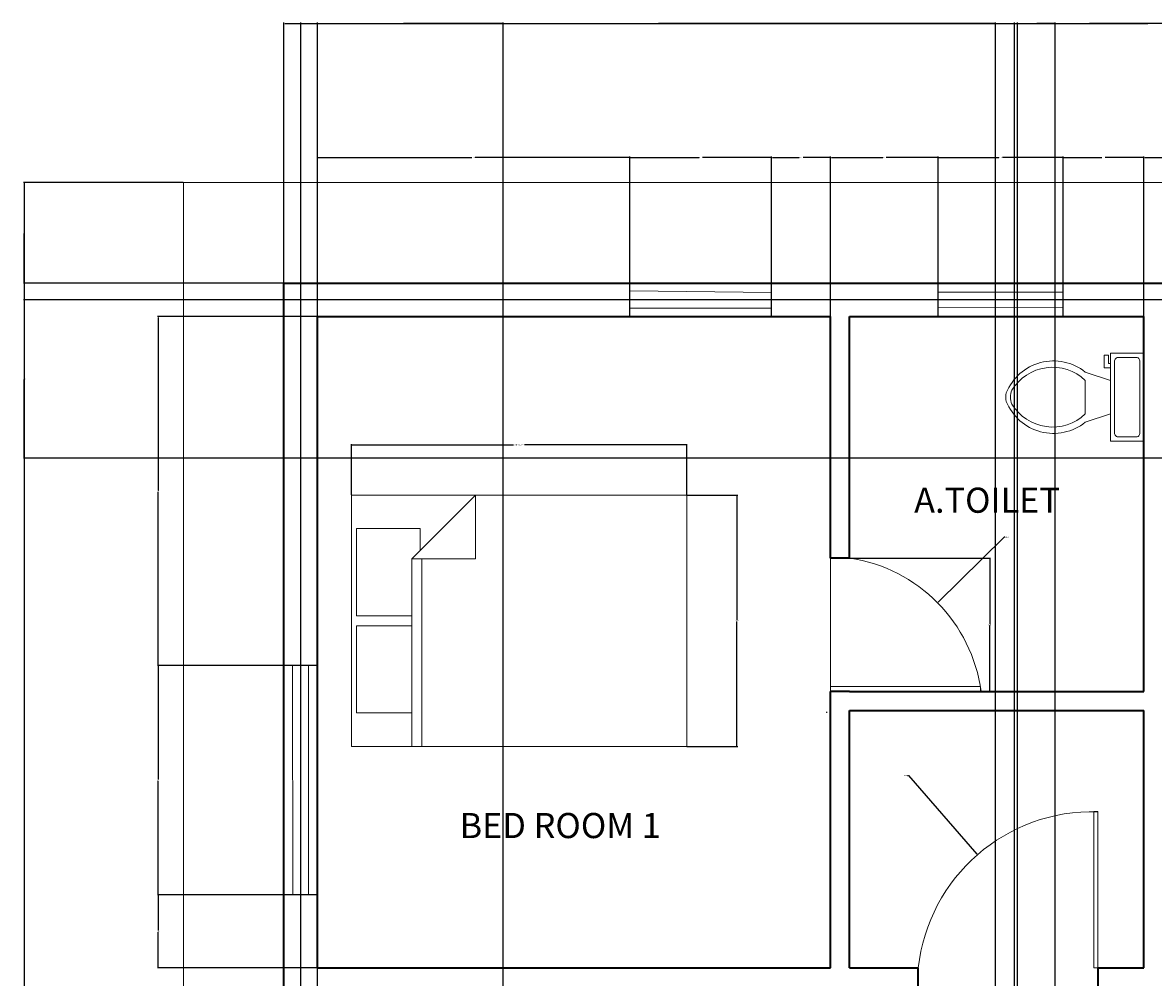
# Model space of a CAD drawing. Units: inches. Extents: x 4700 to 5209, y 8078 to 8754.
# Tile 4 of 5: x 4700 to 4970, y 8526 to 8754. Entities that reach past the tile are written whole.
import ezdxf

# ---------------------------------------------------------------- set-up
doc = ezdxf.new("R2010")
doc.units = ezdxf.units.IN
for name, color, linetype, lineweight in [('A-ANNO-DIMS', 2, 'Continuous', 18), ('A-AREA-IDEN', 7, 'Continuous', 18), ('A-DOOR', 3, 'Continuous', 18), ('A-FLOR-FIXT', 9, 'Continuous', 18), ('A-FURN', 8, 'Continuous', 18), ('A-GLAZ', 4, 'Continuous', 18), ('A-WALL', 7, 'Continuous', 35), ('C-PROP', 8, 'Continuous', 18)]:
    doc.layers.add(name, color=color, linetype=linetype, lineweight=lineweight)
doc.styles.get("Standard").update_dxf_attribs({"font": 'arial.ttf'})
doc.dimstyles.get("Standard").update_dxf_attribs({"dimtxt": 0.18, "dimasz": 0.18, "dimexe": 0.18, "dimexo": 0.0625, "dimgap": 0.09, "dimtad": 0, "dimtih": 1, "dimtoh": 1, "dimdec": 4, "dimzin": 0, "dimdsep": 46, "dimtxsty": 'Standard', "dimcen": 0.09, "dimadec": 0, "dimazin": 0, "dimtfac": 1, "dimtdec": 4, "dimtofl": 0, "dimtmove": 0, "dimatfit": 3, "dimfxl": 1, "dimtolj": 1, "dimtzin": 0, "dimarcsym": 0})

# ---------------------------------------------------------------- blocks, each defined once
blk = doc.blocks.new('Bed - Queen')
for p, q in [((0, -80.00003), (0, 0)), ((0, 0), (59.99999, 0)), ((59.99999, 0), (59.99999, -80.00003)), ((7.99999, -1.2), (28.79998, -1.2)), ((7.99999, -14.4), (7.99999, -1.2)), ((28.79998, -1.2), (28.79998, -14.4)), ((31.19999, -1.2), (51.99999, -1.2)), ((31.19999, -14.4), (31.19999, -1.2)), ((51.99999, -1.2), (51.99999, -16.4)), ((0, -14.4), (44.8, -14.4)), ((59.99999, -29.6), (44.8, -14.4)), ((44.8, -14.4), (44.8, -29.6)), ((44.8, -16.8), (0, -16.8)), ((51.99999, -16.4), (46.79936, -16.4)), ((44.8, -29.6), (59.99999, -29.6)), ((59.99999, -80.00003), (0, -80.00003))]:
    blk.add_line(p, q)
blk = doc.blocks.new('Toilet - top')
for p, q in [((9.5, -6), (9.5, -2)), ((-8, -8.5), (-8, -8)), ((-7, -8), (-7, -9.5)), ((-4, -8), (-6, -14)), ((4, -8), (6, -14)), ((-10, -8.5), (-8, -8.5)), ((-10, -9.5), (-10, -8.5)), ((-7, -9.5), (-10, -9.5)), ((4, -14), (-4, -14))]:
    blk.add_line(p, q)
blk.add_lwpolyline([(10.5, -8), (10.5, 0), (-10.5, 0), (-10.5, -8)], close=True)
for points in [[(-9.5, -2), (-9.5, -6)], [(8.5, -1), (-8.5, -1)], [(-8.5, -7), (8.5, -7)]]:
    blk.add_lwpolyline(points)
for centre, radius, start, end in [((-8.62, -1.88), 0.884, 81.8699, 188.1301), ((8.62, -1.88), 0.884, 351.8699, 98.1301), ((-8.62, -6.12), 0.884, 171.8699, 278.1301), ((8.62, -6.12), 0.884, 261.8699, 8.1301), ((3.52, -21.58), 12.17, 141.4691, 247.9714), ((4.2, -21.82), 11.33, 136.3677, 238.9468), ((-3.52, -21.58), 12.17, 292.0284, 38.5307), ((-4.2, -21.82), 11.33, 301.053, 43.6321), ((0, -27.88), 4, 245.7318, 294.2682), ((0, -29), 4, 254.8605, 285.1395)]:
    blk.add_arc(centre, radius, start, end)
blk = doc.blocks.new('*D6')
at = {"layer": 'A-ANNO-DIMS', "color": 0, "lineweight": -2, "transparency": 16777216}
for p, q in [((4778.93, 8641.19), (4778.93, 8653.31)), ((4779.11, 8653.13), (4817.62, 8653.13)), ((4858.75, 8653.13), (4820.23, 8653.13)), ((4858.93, 8641.19), (4858.93, 8653.31))]:
    blk.add_line(p, q, dxfattribs=at)
at = {"layer": 'A-ANNO-DIMS', "color": 0, "transparency": 16777216}
for points in [[(4779.11, 8653.16), (4779.11, 8653.1), (4778.93, 8653.13)], [(4858.75, 8653.16), (4858.75, 8653.1), (4858.93, 8653.13)]]:
    blk.add_solid(points, dxfattribs=at)
at = {"layer": 'Defpoints', "color": 0, "transparency": 16777216}
for p in [(4778.93, 8653.13), (4778.93, 8641.13), (4858.93, 8641.13)]:
    blk.add_point(p, dxfattribs=at)
at = {"layer": 'A-ANNO-DIMS', "color": 0, "transparency": 16777216, "insert": (4818.93, 8653.13), "char_height": 0.18, "attachment_point": 5}
blk.add_mtext('\\A1;QUEEN BED 80 TYP.', dxfattribs=at)
blk = doc.blocks.new('*D7')
at = {"layer": 'A-ANNO-DIMS', "color": 0, "lineweight": -2, "transparency": 16777216}
for p, q in [((4858.99, 8641.13), (4871.11, 8641.13)), ((4870.93, 8640.95), (4870.93, 8611.31)), ((4870.93, 8581.31), (4870.93, 8610.95)), ((4858.99, 8581.13), (4871.11, 8581.13))]:
    blk.add_line(p, q, dxfattribs=at)
at = {"layer": 'A-ANNO-DIMS', "color": 0, "transparency": 16777216}
for points in [[(4870.9, 8640.95), (4870.96, 8640.95), (4870.93, 8641.13)], [(4870.9, 8581.31), (4870.96, 8581.31), (4870.93, 8581.13)]]:
    blk.add_solid(points, dxfattribs=at)
at = {"layer": 'Defpoints', "color": 0, "transparency": 16777216}
for p in [(4858.93, 8641.13), (4870.93, 8641.13), (4858.93, 8581.13)]:
    blk.add_point(p, dxfattribs=at)
at = {"layer": 'A-ANNO-DIMS', "color": 0, "transparency": 16777216, "insert": (4870.93, 8611.13), "char_height": 0.18, "attachment_point": 5}
blk.add_mtext('\\A1;60 TYP.', dxfattribs=at)
blk = doc.blocks.new('*D15')
at = {"layer": 'A-ANNO-DIMS', "color": 0, "lineweight": -2, "transparency": 16777216}
for p, q in [((4738.72, 8715.75), (4700.6, 8715.75)), ((4700.78, 8715.57), (4700.78, 8415.93)), ((4700.78, 8115.93), (4700.78, 8415.57)), ((4738.72, 8115.75), (4700.6, 8115.75))]:
    blk.add_line(p, q, dxfattribs=at)
at = {"layer": 'A-ANNO-DIMS', "color": 0, "transparency": 16777216}
for points in [[(4700.75, 8715.57), (4700.81, 8715.57), (4700.78, 8715.75)], [(4700.75, 8115.93), (4700.81, 8115.93), (4700.78, 8115.75)]]:
    blk.add_solid(points, dxfattribs=at)
at = {"layer": 'Defpoints', "color": 0, "transparency": 16777216}
for p in [(4700.78, 8715.75), (4738.78, 8715.75), (4738.78, 8115.75)]:
    blk.add_point(p, dxfattribs=at)
at = {"layer": 'A-ANNO-DIMS', "color": 0, "transparency": 16777216, "insert": (4700.78, 8415.75), "char_height": 0.18, "attachment_point": 5}
blk.add_mtext('\\A1;600', dxfattribs=at)
blk = doc.blocks.new('*D16')
at = {"layer": 'A-ANNO-DIMS', "color": 0, "lineweight": -2, "transparency": 16777216}
for p, q in [((4762.78, 8691.81), (4762.78, 8753.93)), ((4762.96, 8753.75), (4954.49, 8753.75)), ((5146.6, 8753.75), (4955.07, 8753.75)), ((5146.78, 8691.81), (5146.78, 8753.93))]:
    blk.add_line(p, q, dxfattribs=at)
at = {"layer": 'A-ANNO-DIMS', "color": 0, "transparency": 16777216}
for points in [[(4762.96, 8753.78), (4762.96, 8753.72), (4762.78, 8753.75)], [(5146.6, 8753.78), (5146.6, 8753.72), (5146.78, 8753.75)]]:
    blk.add_solid(points, dxfattribs=at)
at = {"layer": 'Defpoints', "color": 0, "transparency": 16777216}
for p in [(5146.78, 8753.75), (4762.78, 8691.75), (5146.78, 8691.75)]:
    blk.add_point(p, dxfattribs=at)
at = {"layer": 'A-ANNO-DIMS', "color": 0, "transparency": 16777216, "insert": (4954.78, 8753.75), "char_height": 0.18, "attachment_point": 5}
blk.add_mtext('\\A1;384', dxfattribs=at)
blk = doc.blocks.new('*D18')
at = {"layer": 'A-ANNO-DIMS', "color": 0, "lineweight": -2, "transparency": 16777216}
for p, q in [((4770.78, 8683.81), (4770.78, 8721.93)), ((4770.96, 8721.75), (4807.67, 8721.75)), ((4845.16, 8721.75), (4808.46, 8721.75)), ((4845.34, 8683.81), (4845.34, 8721.93))]:
    blk.add_line(p, q, dxfattribs=at)
at = {"layer": 'A-ANNO-DIMS', "color": 0, "transparency": 16777216}
for points in [[(4770.96, 8721.78), (4770.96, 8721.72), (4770.78, 8721.75)], [(4845.16, 8721.78), (4845.16, 8721.72), (4845.34, 8721.75)]]:
    blk.add_solid(points, dxfattribs=at)
at = {"layer": 'Defpoints', "color": 0, "transparency": 16777216}
for p in [(4845.34, 8721.75), (4770.78, 8683.75), (4845.34, 8683.75)]:
    blk.add_point(p, dxfattribs=at)
at = {"layer": 'A-ANNO-DIMS', "color": 0, "transparency": 16777216, "insert": (4808.06, 8721.75), "char_height": 0.18, "attachment_point": 5}
blk.add_mtext('\\A1;74.56', dxfattribs=at)
blk = doc.blocks.new('*D19')
at = {"layer": 'A-ANNO-DIMS', "color": 0, "lineweight": -2, "transparency": 16777216}
for p, q in [((4845.34, 8683.81), (4845.34, 8721.93)), ((4845.52, 8721.75), (4861.87, 8721.75)), ((4879.01, 8721.75), (4862.66, 8721.75)), ((4879.19, 8683.81), (4879.19, 8721.93))]:
    blk.add_line(p, q, dxfattribs=at)
at = {"layer": 'A-ANNO-DIMS', "color": 0, "transparency": 16777216}
for points in [[(4845.52, 8721.78), (4845.52, 8721.72), (4845.34, 8721.75)], [(4879.01, 8721.78), (4879.01, 8721.72), (4879.19, 8721.75)]]:
    blk.add_solid(points, dxfattribs=at)
at = {"layer": 'Defpoints', "color": 0, "transparency": 16777216}
for p in [(4879.19, 8721.75), (4845.34, 8683.75), (4879.19, 8683.75)]:
    blk.add_point(p, dxfattribs=at)
at = {"layer": 'A-ANNO-DIMS', "color": 0, "transparency": 16777216, "insert": (4862.27, 8721.75), "char_height": 0.18, "attachment_point": 5}
blk.add_mtext('\\A1;33.85', dxfattribs=at)
blk = doc.blocks.new('*D20')
at = {"layer": 'A-ANNO-DIMS', "color": 0, "lineweight": -2, "transparency": 16777216}
for p, q in [((4879.19, 8683.81), (4879.19, 8721.93)), ((4879.37, 8721.75), (4885.78, 8721.75)), ((4893.1, 8721.75), (4886.69, 8721.75)), ((4893.28, 8683.81), (4893.28, 8721.93))]:
    blk.add_line(p, q, dxfattribs=at)
at = {"layer": 'A-ANNO-DIMS', "color": 0, "transparency": 16777216}
for points in [[(4879.37, 8721.78), (4879.37, 8721.72), (4879.19, 8721.75)], [(4893.1, 8721.78), (4893.1, 8721.72), (4893.28, 8721.75)]]:
    blk.add_solid(points, dxfattribs=at)
at = {"layer": 'Defpoints', "color": 0, "transparency": 16777216}
for p in [(4893.28, 8721.75), (4879.19, 8683.75), (4893.28, 8683.75)]:
    blk.add_point(p, dxfattribs=at)
at = {"layer": 'A-ANNO-DIMS', "color": 0, "transparency": 16777216, "insert": (4886.24, 8721.75), "char_height": 0.18, "attachment_point": 5}
blk.add_mtext('\\A1;14.089', dxfattribs=at)
blk = doc.blocks.new('*D21')
at = {"layer": 'A-ANNO-DIMS', "color": 0, "lineweight": -2, "transparency": 16777216}
for p, q in [((4893.28, 8683.81), (4893.28, 8721.93)), ((4893.46, 8721.75), (4905.72, 8721.75)), ((4918.78, 8721.75), (4906.51, 8721.75)), ((4918.96, 8683.81), (4918.96, 8721.93))]:
    blk.add_line(p, q, dxfattribs=at)
at = {"layer": 'A-ANNO-DIMS', "color": 0, "transparency": 16777216}
for points in [[(4893.46, 8721.78), (4893.46, 8721.72), (4893.28, 8721.75)], [(4918.78, 8721.78), (4918.78, 8721.72), (4918.96, 8721.75)]]:
    blk.add_solid(points, dxfattribs=at)
at = {"layer": 'Defpoints', "color": 0, "transparency": 16777216}
for p in [(4918.96, 8721.75), (4893.28, 8683.75), (4918.96, 8683.75)]:
    blk.add_point(p, dxfattribs=at)
at = {"layer": 'A-ANNO-DIMS', "color": 0, "transparency": 16777216, "insert": (4906.12, 8721.75), "char_height": 0.18, "attachment_point": 5}
blk.add_mtext('\\A1;25.68', dxfattribs=at)
blk = doc.blocks.new('*D22')
at = {"layer": 'A-ANNO-DIMS', "color": 0, "lineweight": -2, "transparency": 16777216}
for p, q in [((4918.96, 8683.81), (4918.96, 8721.93)), ((4919.14, 8721.75), (4933.41, 8721.75)), ((4948.61, 8721.75), (4934.34, 8721.75)), ((4948.79, 8683.81), (4948.79, 8721.93))]:
    blk.add_line(p, q, dxfattribs=at)
at = {"layer": 'A-ANNO-DIMS', "color": 0, "transparency": 16777216}
for points in [[(4919.14, 8721.78), (4919.14, 8721.72), (4918.96, 8721.75)], [(4948.61, 8721.78), (4948.61, 8721.72), (4948.79, 8721.75)]]:
    blk.add_solid(points, dxfattribs=at)
at = {"layer": 'Defpoints', "color": 0, "transparency": 16777216}
for p in [(4948.79, 8721.75), (4918.96, 8683.75), (4948.79, 8683.75)]:
    blk.add_point(p, dxfattribs=at)
at = {"layer": 'A-ANNO-DIMS', "color": 0, "transparency": 16777216, "insert": (4933.87, 8721.75), "char_height": 0.18, "attachment_point": 5}
blk.add_mtext('\\A1;29.834', dxfattribs=at)
blk = doc.blocks.new('*D23')
at = {"layer": 'A-ANNO-DIMS', "color": 0, "lineweight": -2, "transparency": 16777216}
for p, q in [((4948.79, 8683.81), (4948.79, 8721.93)), ((4948.97, 8721.75), (4958.05, 8721.75)), ((4967.89, 8721.75), (4958.82, 8721.75)), ((4968.07, 8683.81), (4968.07, 8721.93))]:
    blk.add_line(p, q, dxfattribs=at)
at = {"layer": 'A-ANNO-DIMS', "color": 0, "transparency": 16777216}
for points in [[(4948.97, 8721.78), (4948.97, 8721.72), (4948.79, 8721.75)], [(4967.89, 8721.78), (4967.89, 8721.72), (4968.07, 8721.75)]]:
    blk.add_solid(points, dxfattribs=at)
at = {"layer": 'Defpoints', "color": 0, "transparency": 16777216}
for p in [(4968.07, 8721.75), (4948.79, 8683.75), (4968.07, 8683.75)]:
    blk.add_point(p, dxfattribs=at)
at = {"layer": 'A-ANNO-DIMS', "color": 0, "transparency": 16777216, "insert": (4958.43, 8721.75), "char_height": 0.18, "attachment_point": 5}
blk.add_mtext('\\A1;19.28', dxfattribs=at)
blk = doc.blocks.new('*D24')
at = {"layer": 'A-ANNO-DIMS', "color": 0, "lineweight": -2, "transparency": 16777216}
for p, q in [((4968.07, 8683.81), (4968.07, 8721.93)), ((4968.25, 8721.75), (4979.68, 8721.75)), ((4992.05, 8721.75), (4980.61, 8721.75)), ((4992.23, 8683.81), (4992.23, 8721.93))]:
    blk.add_line(p, q, dxfattribs=at)
at = {"layer": 'A-ANNO-DIMS', "color": 0, "transparency": 16777216}
for points in [[(4968.25, 8721.78), (4968.25, 8721.72), (4968.07, 8721.75)], [(4992.05, 8721.78), (4992.05, 8721.72), (4992.23, 8721.75)]]:
    blk.add_solid(points, dxfattribs=at)
at = {"layer": 'Defpoints', "color": 0, "transparency": 16777216}
for p in [(4992.23, 8721.75), (4968.07, 8683.75), (4992.23, 8683.75)]:
    blk.add_point(p, dxfattribs=at)
at = {"layer": 'A-ANNO-DIMS', "color": 0, "transparency": 16777216, "insert": (4980.15, 8721.75), "char_height": 0.18, "attachment_point": 5}
blk.add_mtext('\\A1;24.153', dxfattribs=at)
blk = doc.blocks.new('*D35')
at = {"layer": 'A-ANNO-DIMS', "color": 0, "lineweight": -2, "transparency": 16777216}
for p, q in [((4770.72, 8545.71), (4732.6, 8545.71)), ((4732.78, 8545.53), (4732.78, 8537.16)), ((4732.78, 8528.43), (4732.78, 8536.8)), ((4770.72, 8528.25), (4732.6, 8528.25))]:
    blk.add_line(p, q, dxfattribs=at)
at = {"layer": 'A-ANNO-DIMS', "color": 0, "transparency": 16777216}
for points in [[(4732.75, 8545.53), (4732.81, 8545.53), (4732.78, 8545.71)], [(4732.75, 8528.43), (4732.81, 8528.43), (4732.78, 8528.25)]]:
    blk.add_solid(points, dxfattribs=at)
at = {"layer": 'Defpoints', "color": 0, "transparency": 16777216}
for p in [(4732.78, 8545.71), (4770.78, 8545.71), (4770.78, 8528.25)]:
    blk.add_point(p, dxfattribs=at)
at = {"layer": 'A-ANNO-DIMS', "color": 0, "transparency": 16777216, "insert": (4732.78, 8536.98), "char_height": 0.18, "attachment_point": 5}
blk.add_mtext('\\A1;17.463', dxfattribs=at)
blk = doc.blocks.new('*D36')
at = {"layer": 'A-ANNO-DIMS', "color": 0, "lineweight": -2, "transparency": 16777216}
for p, q in [((4770.72, 8600.44), (4732.6, 8600.44)), ((4732.78, 8600.26), (4732.78, 8573.26)), ((4732.78, 8545.89), (4732.78, 8572.89)), ((4770.72, 8545.71), (4732.6, 8545.71))]:
    blk.add_line(p, q, dxfattribs=at)
at = {"layer": 'A-ANNO-DIMS', "color": 0, "transparency": 16777216}
for points in [[(4732.75, 8600.26), (4732.81, 8600.26), (4732.78, 8600.44)], [(4732.75, 8545.89), (4732.81, 8545.89), (4732.78, 8545.71)]]:
    blk.add_solid(points, dxfattribs=at)
at = {"layer": 'Defpoints', "color": 0, "transparency": 16777216}
for p in [(4732.78, 8600.44), (4770.78, 8600.44), (4770.78, 8545.71)]:
    blk.add_point(p, dxfattribs=at)
at = {"layer": 'A-ANNO-DIMS', "color": 0, "transparency": 16777216, "insert": (4732.78, 8573.07), "char_height": 0.18, "attachment_point": 5}
blk.add_mtext('\\A1;54.72', dxfattribs=at)
blk = doc.blocks.new('*D37')
at = {"layer": 'A-ANNO-DIMS', "color": 0, "lineweight": -2, "transparency": 16777216}
for p, q in [((4770.72, 8683.75), (4732.6, 8683.75)), ((4732.78, 8683.57), (4732.78, 8642.27)), ((4732.78, 8600.62), (4732.78, 8641.91)), ((4770.72, 8600.44), (4732.6, 8600.44))]:
    blk.add_line(p, q, dxfattribs=at)
at = {"layer": 'A-ANNO-DIMS', "color": 0, "transparency": 16777216}
for points in [[(4732.75, 8683.57), (4732.81, 8683.57), (4732.78, 8683.75)], [(4732.75, 8600.62), (4732.81, 8600.62), (4732.78, 8600.44)]]:
    blk.add_solid(points, dxfattribs=at)
at = {"layer": 'Defpoints', "color": 0, "transparency": 16777216}
for p in [(4732.78, 8683.75), (4770.78, 8683.75), (4770.78, 8600.44)]:
    blk.add_point(p, dxfattribs=at)
at = {"layer": 'A-ANNO-DIMS', "color": 0, "transparency": 16777216, "insert": (4732.78, 8642.09), "char_height": 0.18, "attachment_point": 5}
blk.add_mtext('\\A1;83.32', dxfattribs=at)
blk = doc.blocks.new('*D47')
at = {"layer": 'A-ANNO-DIMS', "color": 0, "lineweight": -2, "transparency": 16777216}
for p, q in [((5142.99, 8687.75), (4700.6, 8687.75)), ((4700.78, 8687.57), (4700.78, 8669.03)), ((4700.78, 8650.12), (4700.78, 8668.66)), ((5142.99, 8649.94), (4700.6, 8649.94))]:
    blk.add_line(p, q, dxfattribs=at)
at = {"layer": 'A-ANNO-DIMS', "color": 0, "transparency": 16777216}
for points in [[(4700.75, 8687.57), (4700.81, 8687.57), (4700.78, 8687.75)], [(4700.75, 8650.12), (4700.81, 8650.12), (4700.78, 8649.94)]]:
    blk.add_solid(points, dxfattribs=at)
at = {"layer": 'Defpoints', "color": 0, "transparency": 16777216}
for p in [(5143.05, 8687.75), (4700.78, 8649.94), (5143.05, 8649.94)]:
    blk.add_point(p, dxfattribs=at)
at = {"layer": 'A-ANNO-DIMS', "color": 0, "transparency": 16777216, "insert": (4700.78, 8668.84), "char_height": 0.18, "attachment_point": 5}
blk.add_mtext('\\A1;37.814', dxfattribs=at)
blk = doc.blocks.new('*D49')
at = {"layer": 'A-ANNO-DIMS', "color": 0, "lineweight": -2, "transparency": 16777216}
for p, q in [((4766.78, 8318.91), (4766.78, 8753.93)), ((4766.96, 8753.75), (4790.57, 8753.75)), ((4814.97, 8753.75), (4791.36, 8753.75)), ((4815.15, 8318.91), (4815.15, 8753.93))]:
    blk.add_line(p, q, dxfattribs=at)
at = {"layer": 'A-ANNO-DIMS', "color": 0, "transparency": 16777216}
for points in [[(4766.96, 8753.78), (4766.96, 8753.72), (4766.78, 8753.75)], [(4814.97, 8753.78), (4814.97, 8753.72), (4815.15, 8753.75)]]:
    blk.add_solid(points, dxfattribs=at)
at = {"layer": 'Defpoints', "color": 0, "transparency": 16777216}
for p in [(4815.15, 8753.75), (4766.78, 8318.85), (4815.15, 8318.85)]:
    blk.add_point(p, dxfattribs=at)
at = {"layer": 'A-ANNO-DIMS', "color": 0, "transparency": 16777216, "insert": (4790.96, 8753.75), "char_height": 0.18, "attachment_point": 5}
blk.add_mtext('\\A1;48.37', dxfattribs=at)
blk = doc.blocks.new('*D51')
at = {"layer": 'A-ANNO-DIMS', "color": 0, "lineweight": -2, "transparency": 16777216}
for p, q in [((4770.78, 8207.81), (4770.78, 8753.93)), ((4770.96, 8753.75), (4851.26, 8753.75)), ((4932.47, 8753.75), (4852.17, 8753.75)), ((4932.65, 8207.81), (4932.65, 8753.93))]:
    blk.add_line(p, q, dxfattribs=at)
at = {"layer": 'A-ANNO-DIMS', "color": 0, "transparency": 16777216}
for points in [[(4770.96, 8753.78), (4770.96, 8753.72), (4770.78, 8753.75)], [(4932.47, 8753.78), (4932.47, 8753.72), (4932.65, 8753.75)]]:
    blk.add_solid(points, dxfattribs=at)
at = {"layer": 'Defpoints', "color": 0, "transparency": 16777216}
for p in [(4932.65, 8753.75), (4770.78, 8207.75), (4932.65, 8207.75)]:
    blk.add_point(p, dxfattribs=at)
at = {"layer": 'A-ANNO-DIMS', "color": 0, "transparency": 16777216, "insert": (4851.71, 8753.75), "char_height": 0.18, "attachment_point": 5}
blk.add_mtext('\\A1;161.87', dxfattribs=at)
blk = doc.blocks.new('*D55')
at = {"layer": 'A-ANNO-DIMS', "color": 0, "lineweight": -2, "transparency": 16777216}
for p, q in [((4937.15, 8207.81), (4937.15, 8753.93)), ((4937.33, 8753.75), (4969.02, 8753.75)), ((5001.49, 8753.75), (4969.8, 8753.75)), ((5001.67, 8207.81), (5001.67, 8753.93))]:
    blk.add_line(p, q, dxfattribs=at)
at = {"layer": 'A-ANNO-DIMS', "color": 0, "transparency": 16777216}
for points in [[(4937.33, 8753.78), (4937.33, 8753.72), (4937.15, 8753.75)], [(5001.49, 8753.78), (5001.49, 8753.72), (5001.67, 8753.75)]]:
    blk.add_solid(points, dxfattribs=at)
at = {"layer": 'Defpoints', "color": 0, "transparency": 16777216}
for p in [(5001.67, 8753.75), (4937.15, 8207.75), (5001.67, 8207.75)]:
    blk.add_point(p, dxfattribs=at)
at = {"layer": 'A-ANNO-DIMS', "color": 0, "transparency": 16777216, "insert": (4969.41, 8753.75), "char_height": 0.18, "attachment_point": 5}
blk.add_mtext('\\A1;64.53', dxfattribs=at)
blk = doc.blocks.new('*D62')
at = {"layer": 'A-ANNO-DIMS', "color": 0, "lineweight": -2, "transparency": 16777216}
for p, q in [((4937.87, 8162.31), (4937.87, 8753.93)), ((4938.05, 8753.75), (4942.22, 8753.75)), ((4946.69, 8753.75), (4942.52, 8753.75)), ((4946.87, 8162.31), (4946.87, 8753.93))]:
    blk.add_line(p, q, dxfattribs=at)
at = {"layer": 'A-ANNO-DIMS', "color": 0, "transparency": 16777216}
for points in [[(4938.05, 8753.78), (4938.05, 8753.72), (4937.87, 8753.75)], [(4946.69, 8753.78), (4946.69, 8753.72), (4946.87, 8753.75)]]:
    blk.add_solid(points, dxfattribs=at)
at = {"layer": 'Defpoints', "color": 0, "transparency": 16777216}
for p in [(4946.87, 8753.75), (4937.87, 8162.25), (4946.87, 8162.25)]:
    blk.add_point(p, dxfattribs=at)
at = {"layer": 'A-ANNO-DIMS', "color": 0, "transparency": 16777216, "insert": (4942.37, 8753.75), "char_height": 0.18, "attachment_point": 5}
blk.add_mtext('\\A1;9', dxfattribs=at)
blk = doc.blocks.new('*D67')
at = {"layer": 'A-ANNO-DIMS', "color": 0, "lineweight": -2, "transparency": 16777216}
for p, q in [((4893.34, 8626.1), (4931.46, 8626.1)), ((4931.28, 8625.92), (4931.28, 8610.36)), ((4931.28, 8594.43), (4931.28, 8609.99)), ((4893.34, 8594.25), (4931.46, 8594.25))]:
    blk.add_line(p, q, dxfattribs=at)
at = {"layer": 'A-ANNO-DIMS', "color": 0, "transparency": 16777216}
for points in [[(4931.25, 8625.92), (4931.31, 8625.92), (4931.28, 8626.1)], [(4931.25, 8594.43), (4931.31, 8594.43), (4931.28, 8594.25)]]:
    blk.add_solid(points, dxfattribs=at)
at = {"layer": 'Defpoints', "color": 0, "transparency": 16777216}
for p in [(4893.28, 8626.1), (4893.28, 8594.25), (4931.28, 8594.25)]:
    blk.add_point(p, dxfattribs=at)
at = {"layer": 'A-ANNO-DIMS', "color": 0, "transparency": 16777216, "insert": (4931.28, 8610.17), "char_height": 0.18, "attachment_point": 5}
blk.add_mtext('\\A1;31.85', dxfattribs=at)
blk = doc.blocks.new('*D74')
at = {"layer": 'A-ANNO-DIMS', "color": 0, "lineweight": -2, "transparency": 16777216}
for p, q in [((4738.72, 8715.75), (4700.6, 8715.75)), ((4700.78, 8715.57), (4700.78, 8703.93)), ((4700.78, 8691.93), (4700.78, 8703.57)), ((4762.72, 8691.75), (4700.6, 8691.75))]:
    blk.add_line(p, q, dxfattribs=at)
at = {"layer": 'A-ANNO-DIMS', "color": 0, "transparency": 16777216}
for points in [[(4700.75, 8715.57), (4700.81, 8715.57), (4700.78, 8715.75)], [(4700.75, 8691.93), (4700.81, 8691.93), (4700.78, 8691.75)]]:
    blk.add_solid(points, dxfattribs=at)
at = {"layer": 'Defpoints', "color": 0, "transparency": 16777216}
for p in [(4700.78, 8715.75), (4738.78, 8715.75), (4762.78, 8691.75)]:
    blk.add_point(p, dxfattribs=at)
at = {"layer": 'A-ANNO-DIMS', "color": 0, "transparency": 16777216, "insert": (4700.78, 8703.75), "char_height": 0.18, "attachment_point": 5}
blk.add_mtext('\\A1;24', dxfattribs=at)
blk = doc.blocks.new('*D79')
at = {"layer": 'A-ANNO-DIMS', "color": 0, "lineweight": -2, "transparency": 16777216}
for p, q in [((4911.66, 8574.22), (4911.84, 8574.22)), ((4911.84, 8574.22), (4928.21, 8555.41)), ((4955.72, 8523.7), (4955.9, 8523.7)), ((4955.81, 8523.61), (4955.81, 8523.79))]:
    blk.add_line(p, q, dxfattribs=at)
at = {"layer": 'A-ANNO-DIMS', "color": 0, "transparency": 16777216}
blk.add_solid([(4928.24, 8555.43), (4928.19, 8555.39), (4928.33, 8555.28)], dxfattribs=at)
at = {"layer": 'Defpoints', "color": 0, "transparency": 16777216}
for p in [(4928.33, 8555.28), (4955.81, 8523.7)]:
    blk.add_point(p, dxfattribs=at)
at = {"layer": 'A-ANNO-DIMS', "color": 0, "transparency": 16777216, "insert": (4911.18, 8574.22), "char_height": 0.18, "attachment_point": 5}
blk.add_mtext('\\A1;R41.86', dxfattribs=at)
blk = doc.blocks.new('*D80')
at = {"layer": 'A-ANNO-DIMS', "color": 0, "lineweight": -2, "transparency": 16777216}
for p, q in [((4934.7, 8631.09), (4918.94, 8615.55)), ((4934.88, 8631.09), (4934.7, 8631.09)), ((4892.26, 8589.32), (4892.44, 8589.32)), ((4892.35, 8589.23), (4892.35, 8589.41))]:
    blk.add_line(p, q, dxfattribs=at)
at = {"layer": 'A-ANNO-DIMS', "color": 0, "transparency": 16777216}
blk.add_solid([(4918.92, 8615.58), (4918.96, 8615.53), (4918.81, 8615.43)], dxfattribs=at)
at = {"layer": 'Defpoints', "color": 0, "transparency": 16777216}
for p in [(4918.81, 8615.43), (4892.35, 8589.32)]:
    blk.add_point(p, dxfattribs=at)
at = {"layer": 'A-ANNO-DIMS', "color": 0, "transparency": 16777216, "insert": (4935.36, 8631.09), "char_height": 0.18, "attachment_point": 5}
blk.add_mtext('\\A1;R37.18', dxfattribs=at)

msp = doc.modelspace()

# ---------------------------------------------------------------- linework, layer by layer
at = {"layer": 'A-DOOR'}
for p, q in [((4893.2803, 8626.0977), (4893.2803, 8595.4376)), ((4893.2803, 8594.2503), (4893.2803, 8595.4376)), ((4893.2803, 8595.4376), (4929.0186, 8595.4376)), ((4929.0186, 8595.4376), (4929.0186, 8594.2503)), ((4957.0498, 8565.5623), (4956.0881, 8565.5623)), ((4956.0881, 8565.5623), (4956.0881, 8528.2503)), ((4957.0498, 8528.2503), (4957.0498, 8565.5623)), ((4956.0881, 8528.2503), (4957.0498, 8528.2503))]:
    msp.add_line(p, q, dxfattribs=at)
for centre, radius, start, end in [((4892.3465, 8589.3177), 37.1792, 7.624037, 81.595939), ((4955.8142, 8523.7042), 41.859, 88.30849, 173.765006)]:
    msp.add_arc(centre, radius, start, end, dxfattribs=at)
at = {"layer": 'A-GLAZ'}
for p, q in [((4845.3443, 8689.9378), (4879.1918, 8689.4962)), ((4918.958, 8689.6078), (4948.7917, 8689.6078)), ((4845.3443, 8687.7503), (4879.1918, 8687.7503)), ((4918.958, 8687.7503), (4948.7917, 8687.7503)), ((4918.958, 8686.0122), (4948.7917, 8685.8462)), ((4845.3443, 8685.7983), (4879.1918, 8685.7983)), ((4764.802, 8600.4352), (4764.943, 8545.7134)), ((4766.7803, 8600.4352), (4766.7803, 8545.7134)), ((4768.6094, 8600.4352), (4768.6094, 8545.7134))]:
    msp.add_line(p, q, dxfattribs=at)
for points in [[(4845.3443, 8691.7503), (4879.1918, 8691.7503), (4879.1918, 8683.7503), (4845.3443, 8683.7503)], [(4918.958, 8691.7503), (4948.7917, 8691.7503), (4948.7917, 8683.7503), (4918.958, 8683.7503)], [(4762.7803, 8600.4352), (4770.7803, 8600.4352), (4770.7803, 8545.7134), (4762.7803, 8545.7134)]]:
    msp.add_lwpolyline(points, close=True, dxfattribs=at)
at = {"layer": 'A-WALL'}
for p, q in [((4762.7803, 8199.7503), (4762.7803, 8691.7503)), ((4762.7803, 8691.7503), (5146.7803, 8691.7503)), ((4770.7803, 8683.7503), (4893.2803, 8683.7503)), ((4770.7803, 8528.2503), (4770.7803, 8683.7503)), ((4893.2803, 8626.0977), (4893.2803, 8683.7503)), ((4897.7803, 8626.0977), (4897.7803, 8683.7503)), ((4897.7803, 8683.7503), (4968.0733, 8683.7503)), ((4968.0733, 8594.2503), (4968.0733, 8683.7503)), ((4897.7803, 8626.0977), (4893.2803, 8626.0977)), ((4893.2803, 8528.2503), (4893.2803, 8594.2503)), ((4897.7803, 8594.2503), (4893.2803, 8594.2503)), ((4897.7803, 8594.2503), (4968.0733, 8594.2503)), ((4897.7803, 8528.2503), (4897.7803, 8589.7503)), ((4897.7803, 8589.7503), (4968.0733, 8589.7503)), ((4968.0733, 8528.2503), (4968.0733, 8589.7503)), ((4770.7803, 8528.2503), (4893.2803, 8528.2503)), ((4897.7803, 8528.2503), (4914.2028, 8528.2503)), ((4914.2028, 8523.7503), (4914.2028, 8528.2503)), ((4957.0498, 8528.2503), (4968.0733, 8528.2503)), ((4957.0498, 8528.2503), (4957.0498, 8523.7503))]:
    msp.add_line(p, q, dxfattribs=at)
at = {"layer": 'C-PROP'}
for p, q in [((4738.7803, 8715.7503), (5170.7803, 8715.7503)), ((4738.7803, 8115.7503), (4738.7803, 8715.7503))]:
    msp.add_line(p, q, dxfattribs=at)

# ---------------------------------------------------------------- block references
at = {"layer": 'A-FLOR-FIXT', "rotation": 270}
msp.add_blockref('Toilet - top', (4968.0733, 8664.5172), dxfattribs=at)
at = {"layer": 'A-FURN', "rotation": 90}
msp.add_blockref('Bed - Queen', (4778.9284, 8581.1291), dxfattribs=at)

# ---------------------------------------------------------------- texts
at = {"layer": 'A-AREA-IDEN', "char_height": 6, "attachment_point": 1}
for s, insert in [('\\pxi-3,l4,t4;A.TOILET', (4907.2178, 8642.9175)), ('BED ROOM 1', (4804.7179, 8565.2514))]:
    msp.add_mtext_dynamic_manual_height_columns(s, width=51.756341, gutter_width=12.5, heights=[0], dxfattribs=dict(at, insert=insert))

# ---------------------------------------------------------------- dimensions: what is measured, and where the dimension line sits
at = {"layer": 'A-ANNO-DIMS'}
for base, p1, p2, override, picture, middle in [((5146.7803, 8753.7503), (4762.7803, 8691.7503), (5146.7803, 8691.7503), {"dimdec": 0, "dimlfac": 1, "dimrnd": 0, "dimzin": 0, "dimdsep": 46, "dimlunit": 2}, '*D16', (4954.7803, 8753.7503)), ((4815.1488, 8753.7503), (4766.7803, 8318.8479), (4815.1488, 8318.8479), {"dimdec": 2, "dimlfac": 1, "dimrnd": 0, "dimzin": 0, "dimdsep": 46, "dimlunit": 2}, '*D49', (4790.9646, 8753.7503)), ((4932.6464, 8753.7503), (4770.7803, 8207.7503), (4932.6464, 8207.7503), {"dimdec": 2, "dimlfac": 1, "dimrnd": 0, "dimzin": 0, "dimdsep": 46, "dimlunit": 2}, '*D51', (4851.7134, 8753.7503)), ((5001.6744, 8753.7503), (4937.1464, 8207.7503), (5001.6744, 8207.7503), {"dimdec": 2, "dimlfac": 1, "dimrnd": 0, "dimzin": 0, "dimdsep": 46, "dimlunit": 2}, '*D55', (4969.4104, 8753.7503)), ((4946.8701, 8753.7503), (4937.87, 8162.2503), (4946.8701, 8162.2503), {"dimdec": 0, "dimlfac": 1, "dimrnd": 0, "dimzin": 0, "dimdsep": 46, "dimlunit": 2}, '*D62', (4942.3701, 8753.7503)), ((4879.1918, 8721.7503), (4845.3443, 8683.7503), (4879.1918, 8683.7503), {"dimdec": 2, "dimlfac": 1, "dimrnd": 0, "dimzin": 0, "dimdsep": 46, "dimlunit": 2}, '*D19', (4862.268, 8721.7503)), ((4893.28033, 8721.75034), (4879.19175, 8683.75034), (4893.28033, 8683.75034), {"dimdec": 3, "dimlfac": 1, "dimrnd": 0, "dimzin": 0, "dimdsep": 46, "dimlunit": 2}, '*D20', (4886.23604, 8721.75034)), ((4918.958, 8721.7503), (4893.2803, 8683.7503), (4918.958, 8683.7503), {"dimdec": 2, "dimlfac": 1, "dimrnd": 0, "dimzin": 0, "dimdsep": 46, "dimlunit": 2}, '*D21', (4906.1192, 8721.7503)), ((4948.7917, 8721.7503), (4918.958, 8683.7503), (4948.7917, 8683.7503), {"dimdec": 3, "dimlfac": 1, "dimrnd": 0, "dimzin": 0, "dimdsep": 46, "dimlunit": 2}, '*D22', (4933.8749, 8721.7503)), ((4968.0733, 8721.7503), (4948.7917, 8683.7503), (4968.0733, 8683.7503), {"dimdec": 2, "dimlfac": 1, "dimrnd": 0, "dimzin": 0, "dimdsep": 46, "dimlunit": 2}, '*D23', (4958.4325, 8721.7503)), ((4992.2261, 8721.7503), (4968.0733, 8683.7503), (4992.2261, 8683.7503), {"dimdec": 3, "dimlfac": 1, "dimrnd": 0, "dimzin": 0, "dimdsep": 46, "dimlunit": 2}, '*D24', (4980.1497, 8721.7503))]:
    dim = msp.add_linear_dim(base=base, p1=p1, p2=p2, dimstyle='Standard', override=override, dxfattribs=at)
    dim.commit()
    dim.dimension.update_dxf_attribs({"geometry": picture, "text_midpoint": middle})
for base, p1, p2, angle, override, picture, middle in [((4845.3443, 8721.7503), (4770.7803, 8683.7503), (4845.3443, 8683.7503), 0, {"dimdec": 2, "dimlfac": 1, "dimrnd": 0, "dimzin": 0, "dimdsep": 46, "dimlunit": 2}, '*D18', (4808.0623, 8721.7503)), ((4700.7803, 8715.7503), (4738.7803, 8115.7503), (4738.7803, 8715.7503), 90, {"dimdec": 0, "dimlfac": 1, "dimrnd": 0, "dimzin": 0, "dimdsep": 46, "dimlunit": 2}, '*D15', (4700.7803, 8415.7503)), ((4700.7803, 8715.7503), (4762.7803, 8691.7503), (4738.7803, 8715.7503), 90, {"dimdec": 0, "dimlfac": 1, "dimrnd": 0, "dimzin": 0, "dimdsep": 46, "dimlunit": 2}, '*D74', (4700.7803, 8703.7503)), ((4700.7803, 8649.9364), (5143.0547, 8687.7503), (5143.0547, 8649.9364), 90, {"dimdec": 3, "dimlfac": 1, "dimrnd": 0, "dimzin": 0, "dimdsep": 46, "dimlunit": 2}, '*D47', (4700.7803, 8668.8434)), ((4732.7803, 8683.7503), (4770.7803, 8600.4352), (4770.7803, 8683.7503), 90, {"dimdec": 2, "dimlfac": 1, "dimrnd": 0, "dimzin": 0, "dimdsep": 46, "dimlunit": 2}, '*D37', (4732.7803, 8642.0928)), ((4931.2803, 8594.2503), (4893.2803, 8626.0977), (4893.2803, 8594.2503), 270, {"dimdec": 2, "dimlfac": 1, "dimrnd": 0, "dimzin": 0, "dimdsep": 46, "dimlunit": 2}, '*D67', (4931.2803, 8610.174)), ((4732.7803, 8600.4352), (4770.7803, 8545.7134), (4770.7803, 8600.4352), 90, {"dimdec": 2, "dimlfac": 1, "dimrnd": 0, "dimzin": 0, "dimdsep": 46, "dimlunit": 2}, '*D36', (4732.7803, 8573.0743)), ((4732.7803, 8545.7134), (4770.7803, 8528.2503), (4770.7803, 8545.7134), 90, {"dimdec": 3, "dimlfac": 1, "dimrnd": 0, "dimzin": 0, "dimdsep": 46, "dimlunit": 2}, '*D35', (4732.7803, 8536.9819))]:
    dim = msp.add_linear_dim(base=base, p1=p1, p2=p2, angle=angle, dimstyle='Standard', override=override, dxfattribs=at)
    dim.commit()
    dim.dimension.update_dxf_attribs({"geometry": picture, "text_midpoint": middle})
for base, p1, p2, angle, text, picture, middle in [((4778.9284, 8653.1291), (4858.9284, 8641.1291), (4778.9284, 8641.1291), 180, 'QUEEN BED <> TYP.', '*D6', (4818.9284, 8653.1291)), ((4870.9284, 8641.1291), (4858.9284, 8581.1291), (4858.9284, 8641.1291), 90, '<> TYP.', '*D7', (4870.9284, 8611.1291))]:
    dim = msp.add_linear_dim(base=base, p1=p1, p2=p2, angle=angle, text=text, dimstyle='Standard', override={"dimdec": 0, "dimlfac": 1, "dimrnd": 0, "dimzin": 0, "dimdsep": 46, "dimlunit": 2}, dxfattribs=at)
    dim.commit()
    dim.dimension.update_dxf_attribs({"geometry": picture, "text_midpoint": middle})
for center, mpoint, picture, middle in [((4892.3465, 8589.3177), (4918.8147, 8615.4277), '*D80', (4935.3556, 8631.0937)), ((4955.8142, 8523.7042), (4928.332, 8555.278), '*D79', (4911.1829, 8574.2223))]:
    dim = msp.add_radius_dim(center=center, mpoint=mpoint, dimstyle='Standard', override={"dimdec": 2, "dimlfac": 1, "dimrnd": 0, "dimzin": 0, "dimdsep": 46, "dimlunit": 2}, dxfattribs=at)
    dim.commit()
    dim.dimension.update_dxf_attribs({"geometry": picture, "text_midpoint": middle, "dimtype": 164})

doc.saveas('drawing.dxf')
